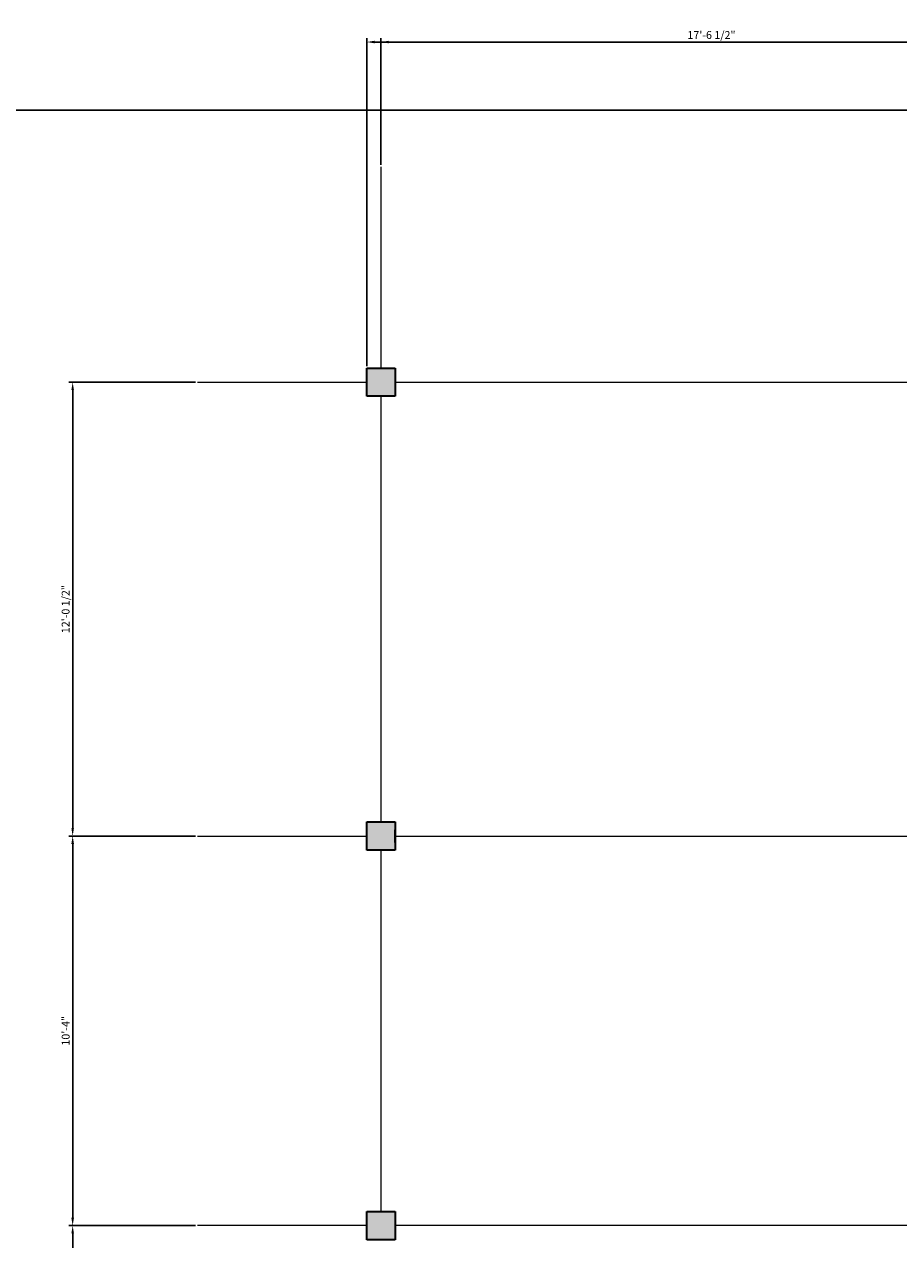
# Model space of a CAD drawing. Units: inches. Extents: x 2169 to 10664, y 1669 to 6352.
# Tile 6 of 17: x 2644 to 2922, y 2479 to 2866. Entities that reach past the tile are written whole.
import ezdxf

# ---------------------------------------------------------------- set-up
doc = ezdxf.new("R2010")
doc.units = ezdxf.units.IN
for name, color, linetype, lineweight in [('A-ANNO-DIMS', 3, 'Continuous', 18), ('A-ANNO-TTLB', 7, 'Continuous', 25), ('A-COLS', 3, 'Continuous', 35), ('A-COLS-PATT', 3, 'Continuous', 13), ('A-GRID', 1, 'Continuous', 13)]:
    doc.layers.add(name, color=color, linetype=linetype, lineweight=lineweight)
doc.styles.get("Standard").update_dxf_attribs({"font": 'arial.ttf'})
doc.dimstyles.new('ISO-25', dxfattribs={"dimtxt": 2.5, "dimasz": 2.5, "dimexe": 1.25, "dimexo": 0.625, "dimtad": 1, "dimdec": 0, "dimlunit": 3, "dimtxsty": 'Standard', "dimcen": 2.5, "dimadec": 0, "dimazin": 0, "dimtfac": 1, "dimtdec": 0, "dimtmove": 0, "dimatfit": 3, "dimfxl": 1, "dimarcsym": 0})

# ---------------------------------------------------------------- blocks, each defined once
blk = doc.blocks.new('COL-9X9')
for p, q in [((0, 9), (9, 9)), ((0, 0), (0, 9)), ((9, 9), (9, 0)), ((9, 0), (0, 0))]:
    blk.add_line(p, q)
blk = doc.blocks.new('*D85')
at = {"layer": 'A-ANNO-DIMS', "color": 0, "lineweight": -2, "transparency": 16777216}
for p, q in [((2757.57, 2820.9), (2757.57, 2861.22)), ((2760.07, 2859.97), (2965.57, 2859.97)), ((2968.07, 2820.9), (2968.07, 2861.22))]:
    blk.add_line(p, q, dxfattribs=at)
at = {"layer": 'A-ANNO-DIMS', "color": 0, "transparency": 16777216}
for points in [[(2760.07, 2860.39), (2760.07, 2859.55), (2757.57, 2859.97)], [(2965.57, 2860.39), (2965.57, 2859.55), (2968.07, 2859.97)]]:
    blk.add_solid(points, dxfattribs=at)
at = {"layer": 'Defpoints', "color": 0, "transparency": 16777216}
for p in [(2968.07, 2859.97), (2757.57, 2820.27), (2968.07, 2820.27)]:
    blk.add_point(p, dxfattribs=at)
at = {"layer": 'A-ANNO-DIMS', "color": 0, "transparency": 16777216, "insert": (2862.82, 2861.89), "char_height": 2.5, "attachment_point": 5}
blk.add_mtext('17\'-6 1/2"', dxfattribs=at)
blk = doc.blocks.new('*D87')
at = {"layer": 'A-ANNO-DIMS', "color": 0, "lineweight": -2, "transparency": 16777216}
for p, q in [((2698.46, 2751.68), (2658.14, 2751.68)), ((2659.39, 2749.18), (2659.39, 2609.68)), ((2698.46, 2607.18), (2658.14, 2607.18))]:
    blk.add_line(p, q, dxfattribs=at)
at = {"layer": 'A-ANNO-DIMS', "color": 0, "transparency": 16777216}
for points in [[(2658.97, 2749.18), (2659.8, 2749.18), (2659.39, 2751.68)], [(2658.97, 2609.68), (2659.8, 2609.68), (2659.39, 2607.18)]]:
    blk.add_solid(points, dxfattribs=at)
at = {"layer": 'Defpoints', "color": 0, "transparency": 16777216}
for p in [(2699.09, 2751.68), (2659.39, 2607.18), (2699.09, 2607.18)]:
    blk.add_point(p, dxfattribs=at)
at = {"layer": 'A-ANNO-DIMS', "color": 0, "transparency": 16777216, "insert": (2657.47, 2679.43), "char_height": 2.5, "attachment_point": 5, "rotation": 90}
blk.add_mtext('12\'-0 1/2"', dxfattribs=at)
blk = doc.blocks.new('*D88')
at = {"layer": 'A-ANNO-DIMS', "color": 0, "lineweight": -2, "transparency": 16777216}
for p, q in [((2698.46, 2607.18), (2658.14, 2607.18)), ((2659.39, 2604.68), (2659.39, 2485.68)), ((2698.46, 2483.18), (2658.14, 2483.18))]:
    blk.add_line(p, q, dxfattribs=at)
at = {"layer": 'A-ANNO-DIMS', "color": 0, "transparency": 16777216}
for points in [[(2658.97, 2604.68), (2659.8, 2604.68), (2659.39, 2607.18)], [(2658.97, 2485.68), (2659.8, 2485.68), (2659.39, 2483.18)]]:
    blk.add_solid(points, dxfattribs=at)
at = {"layer": 'Defpoints', "color": 0, "transparency": 16777216}
for p in [(2699.09, 2607.18), (2659.39, 2483.18), (2699.09, 2483.18)]:
    blk.add_point(p, dxfattribs=at)
at = {"layer": 'A-ANNO-DIMS', "color": 0, "transparency": 16777216, "insert": (2657.49, 2545.18), "char_height": 2.5, "attachment_point": 5, "rotation": 90}
blk.add_mtext('10\'-4"', dxfattribs=at)
blk = doc.blocks.new('*D89')
at = {"layer": 'A-ANNO-DIMS', "color": 0, "lineweight": -2, "transparency": 16777216}
for p, q in [((2698.46, 2483.18), (2658.14, 2483.18)), ((2659.39, 2480.68), (2659.39, 2337.18)), ((2698.46, 2334.68), (2658.14, 2334.68))]:
    blk.add_line(p, q, dxfattribs=at)
at = {"layer": 'A-ANNO-DIMS', "color": 0, "transparency": 16777216}
for points in [[(2658.97, 2480.68), (2659.8, 2480.68), (2659.39, 2483.18)], [(2658.97, 2337.18), (2659.8, 2337.18), (2659.39, 2334.68)]]:
    blk.add_solid(points, dxfattribs=at)
at = {"layer": 'Defpoints', "color": 0, "transparency": 16777216}
for p in [(2699.09, 2483.18), (2659.39, 2334.68), (2699.09, 2334.68)]:
    blk.add_point(p, dxfattribs=at)
at = {"layer": 'A-ANNO-DIMS', "color": 0, "transparency": 16777216, "insert": (2657.47, 2408.93), "char_height": 2.5, "attachment_point": 5, "rotation": 90}
blk.add_mtext('12\'-4 1/2"', dxfattribs=at)
blk = doc.blocks.new('*D91')
at = {"layer": 'A-ANNO-DIMS', "color": 0, "lineweight": -2, "transparency": 16777216}
for p, q in [((2753.07, 2756.81), (2753.07, 2861.22)), ((2755.57, 2859.97), (3110.57, 2859.97)), ((3113.07, 2756.81), (3113.07, 2861.22))]:
    blk.add_line(p, q, dxfattribs=at)
at = {"layer": 'A-ANNO-DIMS', "color": 0, "transparency": 16777216}
for points in [[(2755.57, 2860.39), (2755.57, 2859.55), (2753.07, 2859.97)], [(3110.57, 2860.39), (3110.57, 2859.55), (3113.07, 2859.97)]]:
    blk.add_solid(points, dxfattribs=at)
at = {"layer": 'Defpoints', "color": 0, "transparency": 16777216}
for p in [(3113.07, 2859.97), (2753.07, 2756.18), (3113.07, 2756.18)]:
    blk.add_point(p, dxfattribs=at)
at = {"layer": 'A-ANNO-DIMS', "color": 0, "transparency": 16777216, "insert": (2933.07, 2861.87), "char_height": 2.5, "attachment_point": 5}
blk.add_mtext('30\'-0"', dxfattribs=at)

msp = doc.modelspace()

# ---------------------------------------------------------------- hatches: boundary and pattern name
at = {"layer": 'A-COLS-PATT'}
h = msp.add_hatch(color=256, dxfattribs=at)
h.dxf.hatch_style = 1
h.paths.add_polyline_path([(2762.07, 2165.18), (2753.07, 2165.18), (2753.07, 2156.18), (2762.07, 2156.18)])
h.paths.add_polyline_path([(2972.57, 2165.18), (2963.57, 2165.18), (2963.57, 2156.18), (2972.57, 2156.18)])
h.paths.add_polyline_path([(3113.07, 2165.18), (3104.07, 2165.18), (3104.07, 2156.18), (3113.07, 2156.18)])
h.paths.add_polyline_path([(3113.07, 2330.18), (3113.07, 2339.18), (3104.07, 2339.18), (3104.07, 2330.18)])
h.paths.add_polyline_path([(2972.57, 2339.18), (2963.57, 2339.18), (2963.57, 2330.18), (2972.57, 2330.18)])
h.paths.add_polyline_path([(2762.07, 2330.18), (2762.07, 2339.18), (2753.07, 2339.18), (2753.07, 2330.18)])
h.paths.add_polyline_path([(2753.07, 2478.68), (2762.07, 2478.68), (2762.07, 2487.68), (2753.07, 2487.68)])
h.paths.add_polyline_path([(2963.57, 2487.68), (2963.57, 2478.68), (2972.57, 2478.68), (2972.57, 2487.68)])
h.paths.add_polyline_path([(3104.07, 2487.68), (3104.07, 2478.68), (3113.07, 2478.68), (3113.07, 2487.68)])
h.paths.add_polyline_path([(3104.07, 2602.68), (3113.07, 2602.68), (3113.07, 2611.68), (3104.07, 2611.68)])
h.paths.add_polyline_path([(2963.57, 2602.68), (2972.57, 2602.68), (2972.57, 2611.68), (2963.57, 2611.68)])
h.paths.add_polyline_path([(2753.07, 2611.68), (2753.07, 2602.68), (2762.07, 2602.68), (2762.07, 2611.68)])
h.paths.add_polyline_path([(2762.07, 2747.18), (2762.07, 2756.18), (2753.07, 2756.18), (2753.07, 2747.18)])
h.paths.add_polyline_path([(2972.57, 2747.18), (2972.57, 2756.18), (2963.57, 2756.18), (2963.57, 2747.18)])
h.paths.add_polyline_path([(3104.07, 2756.18), (3104.07, 2747.18), (3113.07, 2747.18), (3113.07, 2756.18)])

# ---------------------------------------------------------------- linework, layer by layer
at = {"layer": 'A-ANNO-TTLB'}
msp.add_lwpolyline([(2169.45, 2838.28), (3251.13, 2838.28), (3251.13, 1669.34), (2169.45, 1669.34)], close=True, dxfattribs=at)
at = {"layer": 'A-COLS'}
msp.add_line((2762.07, 2605.18), (2762.07, 2609.18), dxfattribs=at)
at = {"layer": 'A-GRID'}
for p, q in [((2757.57, 2820.27), (2757.57, 2756.18)), ((2699.09, 2751.68), (2753.07, 2751.68)), ((2762.07, 2751.68), (2963.57, 2751.68)), ((2757.57, 2747.18), (2757.57, 2611.68)), ((2699.09, 2607.18), (2753.07, 2607.18)), ((2762.07, 2607.18), (2963.57, 2607.18)), ((2757.57, 2602.68), (2757.57, 2487.68)), ((2753.07, 2483.18), (2699.09, 2483.18)), ((2963.57, 2483.18), (2762.07, 2483.18))]:
    msp.add_line(p, q, dxfattribs=at)

# ---------------------------------------------------------------- block references
at = {"layer": 'A-COLS'}
msp.add_blockref('COL-9X9', (2753.07, 2747.18), dxfattribs=at)
at = {"layer": 'A-COLS', "rotation": 180}
for p in [(2762.07, 2611.68), (2762.07, 2487.68)]:
    msp.add_blockref('COL-9X9', p, dxfattribs=at)

# ---------------------------------------------------------------- dimensions: what is measured, and where the dimension line sits
at = {"layer": 'A-ANNO-DIMS'}
for base, p1, p2, picture, middle in [((3113.07, 2859.97), (2753.07, 2756.18), (3113.07, 2756.18), '*D91', (2933.07, 2861.87)), ((2968.07, 2859.97), (2757.57, 2820.27), (2968.07, 2820.27), '*D85', (2862.82, 2861.89))]:
    dim = msp.add_linear_dim(base=base, p1=p1, p2=p2, dimstyle='ISO-25', override={"dimdec": 1, "dimlfac": 1, "dimrnd": 0, "dimzin": 1, "dimdsep": 46, "dimlunit": 4, "dimfrac": 2}, dxfattribs=at)
    dim.commit()
    dim.dimension.update_dxf_attribs({"geometry": picture, "text_midpoint": middle})
for base, p1, p2, picture, middle in [((2659.39, 2607.18), (2699.09, 2751.68), (2699.09, 2607.18), '*D87', (2657.47, 2679.43)), ((2659.39, 2483.18), (2699.09, 2607.18), (2699.09, 2483.18), '*D88', (2657.49, 2545.18)), ((2659.39, 2334.68), (2699.09, 2483.18), (2699.09, 2334.68), '*D89', (2657.47, 2408.93))]:
    dim = msp.add_linear_dim(base=base, p1=p1, p2=p2, angle=90, dimstyle='ISO-25', override={"dimdec": 1, "dimlfac": 1, "dimrnd": 0, "dimzin": 1, "dimdsep": 46, "dimlunit": 4, "dimfrac": 2}, dxfattribs=at)
    dim.commit()
    dim.dimension.update_dxf_attribs({"geometry": picture, "text_midpoint": middle})

doc.saveas('drawing.dxf')
